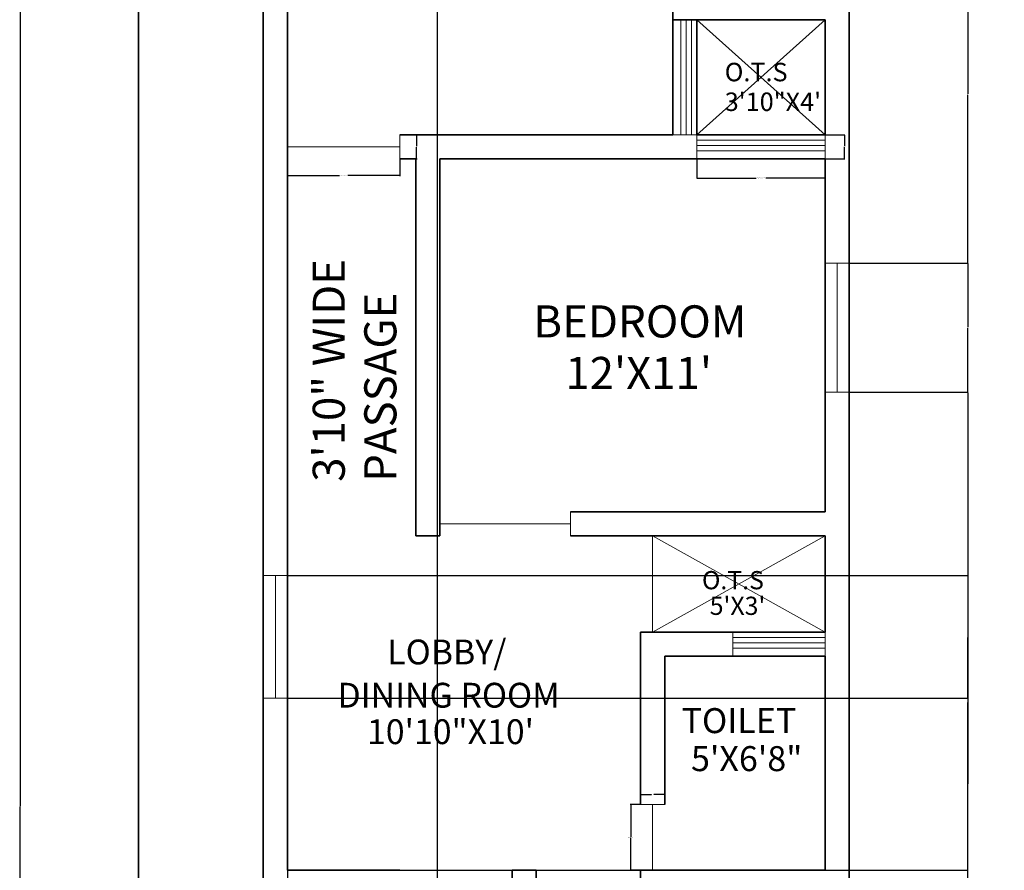
# Model space of a CAD drawing. Units: feet. Extents: x 2100 to 2836, y 2433 to 3396.
# Tile 7 of 12: x 2100 to 2468, y 2906 to 3224. Entities that reach past the tile are written whole.
import ezdxf

# ---------------------------------------------------------------- set-up
doc = ezdxf.new("R2010")
doc.units = ezdxf.units.FT
for name, color, linetype, lineweight in [('A-ANNO-DIMS', 2, 'Continuous', 18), ('A-ANNO-TTLB', 7, 'Continuous', 35), ('A-AREA-IDEN', 7, 'Continuous', 18), ('A-DOOR', 3, 'Continuous', 18), ('A-FLOR-OPEN', 8, 'Continuous', 13), ('A-GLAZ', 4, 'Continuous', 18), ('A-WALL', 7, 'Continuous', 35)]:
    doc.layers.add(name, color=color, linetype=linetype, lineweight=lineweight)
doc.styles.get("Standard").update_dxf_attribs({"font": 'arial.ttf'})
doc.dimstyles.get("Standard").update_dxf_attribs({"dimtxt": 0.18, "dimasz": 0.18, "dimexe": 0.18, "dimexo": 0.0625, "dimgap": 0.09, "dimtad": 0, "dimtih": 1, "dimtoh": 1, "dimdec": 4, "dimzin": 0, "dimdsep": 46, "dimtxsty": 'Standard', "dimcen": 0.09, "dimadec": 0, "dimazin": 0, "dimtfac": 1, "dimtdec": 4, "dimtofl": 0, "dimtmove": 0, "dimatfit": 3, "dimfxl": 1, "dimtolj": 1, "dimtzin": 0, "dimarcsym": 0})

# ---------------------------------------------------------------- blocks, each defined once
blk = doc.blocks.new('OTS-MARK-REAR')
for p, q in [((48, 0), (0, 43)), ((0, 0), (48, 43))]:
    blk.add_line(p, q)
blk = doc.blocks.new('OTS-MARK-LOBBY')
for p, q in [((0, 36), (64.5, 0)), ((0, 0), (64.5, 36))]:
    blk.add_line(p, q)
blk = doc.blocks.new('WIN-TOILET-OTS')
for p, q in [((0, 9), (0, 0)), ((34.5, 9), (34.5, 0)), ((34.5, 7), (0, 7)), ((34.5, 5), (0, 5)), ((34.5, 3), (0, 3))]:
    blk.add_line(p, q)
blk = doc.blocks.new('WIN-BEDROOM-OTS')
for p, q in [((0, 9), (0, 0)), ((48, 9), (48, 0)), ((0, 7), (48, 7)), ((0, 5), (48, 5)), ((0, 3), (48, 3))]:
    blk.add_line(p, q)
blk = doc.blocks.new('WIN-REAR-BEDROOM-OTS')
for p, q in [((3, 43), (3, 0)), ((5, 43), (5, 0)), ((7, 43), (7, 0)), ((0, 0), (9, 0))]:
    blk.add_line(p, q)
blk = doc.blocks.new('DOOR-LOBBY-TOILET')
for p, q in [((0, 24.62), (9, 24.62)), ((4.5, 24.62), (4.5, 0))]:
    blk.add_line(p, q)
blk = doc.blocks.new('DOOR-BEDROOM-LOBBY')
for p, q in [((48.78, 9), (48.78, 0)), ((48.78, 4.5), (0, 4.5))]:
    blk.add_line(p, q)
blk = doc.blocks.new('DOOR-PASSAGE')
for p, q in [((42, 0), (42, 9)), ((42, 4.5), (0, 4.5))]:
    blk.add_line(p, q)
blk = doc.blocks.new('*D16')
at = {"layer": 'A-ANNO-DIMS', "color": 0, "lineweight": -2, "transparency": 16777216}
for p, q in [((2199.69, 3171.74), (2199.69, 3165.32)), ((2241.69, 3171.74), (2241.69, 3165.32)), ((2199.87, 3165.5), (2219.11, 3165.5)), ((2241.51, 3165.5), (2222.26, 3165.5))]:
    blk.add_line(p, q, dxfattribs=at)
at = {"layer": 'A-ANNO-DIMS', "color": 0, "transparency": 16777216}
for points in [[(2199.87, 3165.53), (2199.87, 3165.47), (2199.69, 3165.5)], [(2241.51, 3165.53), (2241.51, 3165.47), (2241.69, 3165.5)]]:
    blk.add_solid(points, dxfattribs=at)
at = {"layer": 'Defpoints', "color": 0, "transparency": 16777216}
for p in [(2199.69, 3171.8), (2241.69, 3171.8), (2241.69, 3165.5)]:
    blk.add_point(p, dxfattribs=at)
at = {"layer": 'A-ANNO-DIMS', "color": 0, "transparency": 16777216, "insert": (2220.69, 3165.5), "char_height": 0.18, "attachment_point": 5}
blk.add_mtext('\\A1;PASSAGE DOOR 42 TYP.', dxfattribs=at)
blk = doc.blocks.new('*D17')
at = {"layer": 'A-ANNO-DIMS', "color": 0, "lineweight": -2, "transparency": 16777216}
for p, q in [((2241.75, 3180.8), (2248.17, 3180.8)), ((2247.99, 3180.62), (2247.99, 3176.48)), ((2247.99, 3171.98), (2247.99, 3176.12)), ((2241.75, 3171.8), (2248.17, 3171.8))]:
    blk.add_line(p, q, dxfattribs=at)
at = {"layer": 'A-ANNO-DIMS', "color": 0, "transparency": 16777216}
for points in [[(2247.96, 3180.62), (2248.02, 3180.62), (2247.99, 3180.8)], [(2247.96, 3171.98), (2248.02, 3171.98), (2247.99, 3171.8)]]:
    blk.add_solid(points, dxfattribs=at)
at = {"layer": 'Defpoints', "color": 0, "transparency": 16777216}
for p in [(2241.69, 3180.8), (2247.99, 3180.8), (2241.69, 3171.8)]:
    blk.add_point(p, dxfattribs=at)
at = {"layer": 'A-ANNO-DIMS', "color": 0, "transparency": 16777216, "insert": (2247.99, 3176.3), "char_height": 0.18, "attachment_point": 5}
blk.add_mtext('\\A1;9 TYP.', dxfattribs=at)
blk = doc.blocks.new('*D26')
at = {"layer": 'A-ANNO-DIMS', "color": 0, "lineweight": -2, "transparency": 16777216}
for p, q in [((2352.69, 3171.74), (2352.69, 3164.42)), ((2400.69, 3171.74), (2400.69, 3164.42)), ((2352.87, 3164.6), (2374.89, 3164.6)), ((2400.51, 3164.6), (2378.48, 3164.6))]:
    blk.add_line(p, q, dxfattribs=at)
at = {"layer": 'A-ANNO-DIMS', "color": 0, "transparency": 16777216}
for points in [[(2352.87, 3164.63), (2352.87, 3164.57), (2352.69, 3164.6)], [(2400.51, 3164.63), (2400.51, 3164.57), (2400.69, 3164.6)]]:
    blk.add_solid(points, dxfattribs=at)
at = {"layer": 'Defpoints', "color": 0, "transparency": 16777216}
for p in [(2352.69, 3171.8), (2400.69, 3171.8), (2400.69, 3164.6)]:
    blk.add_point(p, dxfattribs=at)
at = {"layer": 'A-ANNO-DIMS', "color": 0, "transparency": 16777216, "insert": (2376.69, 3164.6), "char_height": 0.18, "attachment_point": 5}
blk.add_mtext('\\A1;BEDROOM WINDOW 48 TYP.', dxfattribs=at)
blk = doc.blocks.new('*D27')
at = {"layer": 'A-ANNO-DIMS', "color": 0, "lineweight": -2, "transparency": 16777216}
for p, q in [((2400.75, 3180.8), (2408.07, 3180.8)), ((2407.89, 3180.62), (2407.89, 3176.48)), ((2407.89, 3171.98), (2407.89, 3176.12)), ((2400.75, 3171.8), (2408.07, 3171.8))]:
    blk.add_line(p, q, dxfattribs=at)
at = {"layer": 'A-ANNO-DIMS', "color": 0, "transparency": 16777216}
for points in [[(2407.86, 3180.62), (2407.92, 3180.62), (2407.89, 3180.8)], [(2407.86, 3171.98), (2407.92, 3171.98), (2407.89, 3171.8)]]:
    blk.add_solid(points, dxfattribs=at)
at = {"layer": 'Defpoints', "color": 0, "transparency": 16777216}
for p in [(2400.69, 3180.8), (2407.89, 3180.8), (2400.69, 3171.8)]:
    blk.add_point(p, dxfattribs=at)
at = {"layer": 'A-ANNO-DIMS', "color": 0, "transparency": 16777216, "insert": (2407.89, 3176.3), "char_height": 0.18, "attachment_point": 5}
blk.add_mtext('\\A1;9 TYP.', dxfattribs=at)
blk = doc.blocks.new('*D32')
at = {"layer": 'A-ANNO-DIMS', "color": 0, "lineweight": -2, "transparency": 16777216}
for p, q in [((2331.62, 2930.42), (2327.81, 2930.42)), ((2327.99, 2930.24), (2327.99, 2918.29)), ((2327.99, 2905.98), (2327.99, 2917.93)), ((2331.62, 2905.8), (2327.81, 2905.8))]:
    blk.add_line(p, q, dxfattribs=at)
at = {"layer": 'A-ANNO-DIMS', "color": 0, "transparency": 16777216}
for points in [[(2327.96, 2930.24), (2328.02, 2930.24), (2327.99, 2930.42)], [(2327.96, 2905.98), (2328.02, 2905.98), (2327.99, 2905.8)]]:
    blk.add_solid(points, dxfattribs=at)
at = {"layer": 'Defpoints', "color": 0, "transparency": 16777216}
for p in [(2327.99, 2930.42), (2331.69, 2930.42), (2331.69, 2905.8)]:
    blk.add_point(p, dxfattribs=at)
at = {"layer": 'A-ANNO-DIMS', "color": 0, "transparency": 16777216, "insert": (2327.99, 2918.11), "char_height": 0.18, "attachment_point": 5}
blk.add_mtext('\\A1;WC DOOR 25 TYP.', dxfattribs=at)
blk = doc.blocks.new('*D33')
at = {"layer": 'A-ANNO-DIMS', "color": 0, "lineweight": -2, "transparency": 16777216}
for p, q in [((2331.69, 2930.48), (2331.69, 2934.29)), ((2331.87, 2934.11), (2335.73, 2934.11)), ((2340.51, 2934.11), (2336.64, 2934.11)), ((2340.69, 2930.48), (2340.69, 2934.29))]:
    blk.add_line(p, q, dxfattribs=at)
at = {"layer": 'A-ANNO-DIMS', "color": 0, "transparency": 16777216}
for points in [[(2331.87, 2934.14), (2331.87, 2934.08), (2331.69, 2934.11)], [(2340.51, 2934.14), (2340.51, 2934.08), (2340.69, 2934.11)]]:
    blk.add_solid(points, dxfattribs=at)
at = {"layer": 'Defpoints', "color": 0, "transparency": 16777216}
for p in [(2340.69, 2934.11), (2331.69, 2930.42), (2340.69, 2930.42)]:
    blk.add_point(p, dxfattribs=at)
at = {"layer": 'A-ANNO-DIMS', "color": 0, "transparency": 16777216, "insert": (2336.19, 2934.11), "char_height": 0.18, "attachment_point": 5}
blk.add_mtext('\\A1;9 TYP.', dxfattribs=at)
blk = doc.blocks.new('*D41')
at = {"layer": 'A-ANNO-DIMS', "color": 0, "lineweight": -2, "transparency": 16777216}
for p, q in [((2190.62, 3321.8), (2099.65, 3321.8)), ((2099.83, 3321.62), (2099.83, 2929.96)), ((2099.83, 2537.94), (2099.83, 2929.6)), ((2190.62, 2537.76), (2099.65, 2537.76))]:
    blk.add_line(p, q, dxfattribs=at)
at = {"layer": 'A-ANNO-DIMS', "color": 0, "transparency": 16777216}
for points in [[(2099.8, 3321.62), (2099.86, 3321.62), (2099.83, 3321.8)], [(2099.8, 2537.94), (2099.86, 2537.94), (2099.83, 2537.76)]]:
    blk.add_solid(points, dxfattribs=at)
at = {"layer": 'Defpoints', "color": 0, "transparency": 16777216}
for p in [(2099.83, 3321.8), (2190.69, 3321.8), (2190.69, 2537.76)]:
    blk.add_point(p, dxfattribs=at)
at = {"layer": 'A-ANNO-DIMS', "color": 0, "transparency": 16777216, "insert": (2099.83, 2929.78), "char_height": 0.18, "attachment_point": 5}
blk.add_mtext('\\A1;784', dxfattribs=at)
blk = doc.blocks.new('*D44')
at = {"layer": 'A-ANNO-DIMS', "color": 0, "lineweight": -2, "transparency": 16777216}
for p, q in [((2199.69, 3312.74), (2199.69, 2433.01)), ((2255.63, 3312.74), (2255.63, 2433.01)), ((2199.87, 2433.19), (2227.26, 2433.19)), ((2255.45, 2433.19), (2228.05, 2433.19))]:
    blk.add_line(p, q, dxfattribs=at)
at = {"layer": 'A-ANNO-DIMS', "color": 0, "transparency": 16777216}
for points in [[(2199.87, 2433.22), (2199.87, 2433.16), (2199.69, 2433.19)], [(2255.45, 2433.22), (2255.45, 2433.16), (2255.63, 2433.19)]]:
    blk.add_solid(points, dxfattribs=at)
at = {"layer": 'Defpoints', "color": 0, "transparency": 16777216}
for p in [(2199.69, 3312.8), (2255.63, 3312.8), (2255.63, 2433.19)]:
    blk.add_point(p, dxfattribs=at)
at = {"layer": 'A-ANNO-DIMS', "color": 0, "transparency": 16777216, "insert": (2227.66, 2433.19), "char_height": 0.18, "attachment_point": 5}
blk.add_mtext('\\A1;55.94', dxfattribs=at)
blk = doc.blocks.new('*D48')
at = {"layer": 'A-ANNO-DIMS', "color": 0, "lineweight": -2, "transparency": 16777216}
for p, q in [((2409.75, 3259.04), (2454.12, 3259.04)), ((2453.94, 3258.86), (2453.94, 3196.12)), ((2453.94, 3133.01), (2453.94, 3195.75)), ((2409.75, 3132.83), (2454.12, 3132.83))]:
    blk.add_line(p, q, dxfattribs=at)
at = {"layer": 'A-ANNO-DIMS', "color": 0, "transparency": 16777216}
for points in [[(2453.91, 3258.86), (2453.97, 3258.86), (2453.94, 3259.04)], [(2453.91, 3133.01), (2453.97, 3133.01), (2453.94, 3132.83)]]:
    blk.add_solid(points, dxfattribs=at)
at = {"layer": 'Defpoints', "color": 0, "transparency": 16777216}
for p in [(2409.69, 3259.04), (2409.69, 3132.83), (2453.94, 3132.83)]:
    blk.add_point(p, dxfattribs=at)
at = {"layer": 'A-ANNO-DIMS', "color": 0, "transparency": 16777216, "insert": (2453.94, 3195.94), "char_height": 0.18, "attachment_point": 5}
blk.add_mtext('\\A1;126.2', dxfattribs=at)
blk = doc.blocks.new('*D49')
at = {"layer": 'A-ANNO-DIMS', "color": 0, "lineweight": -2, "transparency": 16777216}
for p, q in [((2409.75, 3132.83), (2454.12, 3132.83)), ((2453.94, 3132.65), (2453.94, 3108.87)), ((2453.94, 3084.72), (2453.94, 3108.51)), ((2409.75, 3084.54), (2454.12, 3084.54))]:
    blk.add_line(p, q, dxfattribs=at)
at = {"layer": 'A-ANNO-DIMS', "color": 0, "transparency": 16777216}
for points in [[(2453.91, 3132.65), (2453.97, 3132.65), (2453.94, 3132.83)], [(2453.91, 3084.72), (2453.97, 3084.72), (2453.94, 3084.54)]]:
    blk.add_solid(points, dxfattribs=at)
at = {"layer": 'Defpoints', "color": 0, "transparency": 16777216}
for p in [(2409.69, 3132.83), (2409.69, 3084.54), (2453.94, 3084.54)]:
    blk.add_point(p, dxfattribs=at)
at = {"layer": 'A-ANNO-DIMS', "color": 0, "transparency": 16777216, "insert": (2453.94, 3108.69), "char_height": 0.18, "attachment_point": 5}
blk.add_mtext('\\A1;48.29', dxfattribs=at)
blk = doc.blocks.new('*D50')
at = {"layer": 'A-ANNO-DIMS', "color": 0, "lineweight": -2, "transparency": 16777216}
for p, q in [((2409.75, 3084.54), (2454.12, 3084.54)), ((2453.94, 3084.36), (2453.94, 2968.97)), ((2453.94, 2853.21), (2453.94, 2968.6)), ((2409.75, 2853.03), (2454.12, 2853.03))]:
    blk.add_line(p, q, dxfattribs=at)
at = {"layer": 'A-ANNO-DIMS', "color": 0, "transparency": 16777216}
for points in [[(2453.91, 3084.36), (2453.97, 3084.36), (2453.94, 3084.54)], [(2453.91, 2853.21), (2453.97, 2853.21), (2453.94, 2853.03)]]:
    blk.add_solid(points, dxfattribs=at)
at = {"layer": 'Defpoints', "color": 0, "transparency": 16777216}
for p in [(2409.69, 3084.54), (2409.69, 2853.03), (2453.94, 2853.03)]:
    blk.add_point(p, dxfattribs=at)
at = {"layer": 'A-ANNO-DIMS', "color": 0, "transparency": 16777216, "insert": (2453.94, 2968.78), "char_height": 0.18, "attachment_point": 5}
blk.add_mtext('\\A1;231.5', dxfattribs=at)
blk = doc.blocks.new('*D52')
at = {"layer": 'A-ANNO-DIMS', "color": 0, "lineweight": -2, "transparency": 16777216}
for p, q in [((2199.75, 2970.11), (2454.12, 2970.11)), ((2453.94, 2969.93), (2453.94, 2938.14)), ((2453.94, 2905.98), (2453.94, 2937.78)), ((2199.75, 2905.8), (2454.12, 2905.8))]:
    blk.add_line(p, q, dxfattribs=at)
at = {"layer": 'A-ANNO-DIMS', "color": 0, "transparency": 16777216}
for points in [[(2453.91, 2969.93), (2453.97, 2969.93), (2453.94, 2970.11)], [(2453.91, 2905.98), (2453.97, 2905.98), (2453.94, 2905.8)]]:
    blk.add_solid(points, dxfattribs=at)
at = {"layer": 'Defpoints', "color": 0, "transparency": 16777216}
for p in [(2199.69, 2970.11), (2453.94, 2970.11), (2199.69, 2905.8)]:
    blk.add_point(p, dxfattribs=at)
at = {"layer": 'A-ANNO-DIMS', "color": 0, "transparency": 16777216, "insert": (2453.94, 2937.96), "char_height": 0.18, "attachment_point": 5}
blk.add_mtext('\\A1;64.31', dxfattribs=at)
blk = doc.blocks.new('*D53')
at = {"layer": 'A-ANNO-DIMS', "color": 0, "lineweight": -2, "transparency": 16777216}
for p, q in [((2199.75, 3016.03), (2454.12, 3016.03)), ((2453.94, 3015.85), (2453.94, 2993.26)), ((2453.94, 2970.29), (2453.94, 2992.89)), ((2199.75, 2970.11), (2454.12, 2970.11))]:
    blk.add_line(p, q, dxfattribs=at)
at = {"layer": 'A-ANNO-DIMS', "color": 0, "transparency": 16777216}
for points in [[(2453.91, 3015.85), (2453.97, 3015.85), (2453.94, 3016.03)], [(2453.91, 2970.29), (2453.97, 2970.29), (2453.94, 2970.11)]]:
    blk.add_solid(points, dxfattribs=at)
at = {"layer": 'Defpoints', "color": 0, "transparency": 16777216}
for p in [(2199.69, 3016.03), (2453.94, 3016.03), (2199.69, 2970.11)]:
    blk.add_point(p, dxfattribs=at)
at = {"layer": 'A-ANNO-DIMS', "color": 0, "transparency": 16777216, "insert": (2453.94, 2993.07), "char_height": 0.18, "attachment_point": 5}
blk.add_mtext('\\A1;45.92', dxfattribs=at)

msp = doc.modelspace()

# ---------------------------------------------------------------- linework, layer by layer
at = {"layer": 'A-ANNO-TTLB'}
msp.add_lwpolyline([(2144.0848, 3351.6245), (2791.0561, 3351.6245), (2791.0561, 2477.4373), (2144.0848, 2477.4373)], close=True, dxfattribs=at)
at = {"layer": 'A-FLOR-OPEN'}
msp.add_line((2336.1857, 2994.8031), (2336.1857, 3030.8031), dxfattribs=at)
at = {"layer": 'A-GLAZ'}
for p, q in [((2400.6857, 3132.8348), (2409.6857, 3132.8348)), ((2405.1857, 3084.5411), (2405.1857, 3132.8348)), ((2400.6857, 3084.5411), (2409.6857, 3084.5411)), ((2190.6857, 3016.035), (2199.6857, 3016.035)), ((2195.1857, 2970.1128), (2195.1857, 3016.035)), ((2190.6857, 2970.1128), (2199.6857, 2970.1128))]:
    msp.add_line(p, q, dxfattribs=at)
at = {"layer": 'A-WALL'}
for p, q in [((2190.6857, 2593.755), (2190.6857, 3321.8031)), ((2409.6857, 3321.8031), (2409.6857, 3171.8031)), ((2199.6857, 2905.8031), (2199.6857, 3312.8031)), ((2343.6857, 3260.1235), (2343.6857, 3180.8031)), ((2400.6857, 3223.8031), (2343.6857, 3223.8031)), ((2352.6857, 3223.8031), (2352.6857, 3180.8031)), ((2352.6857, 3223.8031), (2352.6857, 3180.8031)), ((2352.6857, 3223.8031), (2352.6857, 3180.8031)), ((2352.6857, 3223.8031), (2400.6857, 3223.8031)), ((2352.6857, 3223.8031), (2396.5765, 3223.8031)), ((2400.6857, 3223.8031), (2400.6857, 3180.8031)), ((2343.6857, 3180.8031), (2241.6857, 3180.8031)), ((2352.6857, 3180.8031), (2400.6857, 3180.8031)), ((2247.6857, 3171.8031), (2241.6857, 3171.8031)), ((2247.6857, 3171.8031), (2247.6857, 3039.8031)), ((2400.6857, 3171.8031), (2256.6857, 3171.8031)), ((2256.6857, 3171.8031), (2256.6857, 3030.8031)), ((2400.6857, 3039.8031), (2400.6857, 3171.8031)), ((2409.6857, 3171.8031), (2409.6857, 2987.2733)), ((2247.6857, 3039.8031), (2247.6857, 3030.8031)), ((2305.4641, 3039.8031), (2400.6857, 3039.8031)), ((2247.6857, 3030.8031), (2256.6857, 3030.8031)), ((2305.4641, 3030.8031), (2400.6857, 3030.8031)), ((2400.6857, 3030.8031), (2400.6857, 2994.8031)), ((2400.6857, 2994.8031), (2331.6857, 2994.8031)), ((2331.6857, 2994.8031), (2331.6857, 2930.4198)), ((2400.6857, 2985.8031), (2340.6857, 2985.8031)), ((2340.6857, 2985.8031), (2340.6857, 2930.4198)), ((2400.6857, 2905.8031), (2400.6857, 2985.8031)), ((2409.6857, 2987.2733), (2409.6857, 2891.1053)), ((2241.6857, 2905.8031), (2199.6857, 2905.8031)), ((2283.6857, 2905.8031), (2292.6857, 2905.8031)), ((2283.6857, 2810.8031), (2283.6857, 2905.8031)), ((2292.6857, 2801.8031), (2292.6857, 2905.8031)), ((2331.6857, 2905.8031), (2331.6857, 2896.8031)), ((2331.6857, 2905.8031), (2400.6857, 2905.8031))]:
    msp.add_line(p, q, dxfattribs=at)

# ---------------------------------------------------------------- block references
at = {"layer": 'A-DOOR'}
for name, p in [('DOOR-PASSAGE', (2199.6857, 3171.8031)), ('DOOR-BEDROOM-LOBBY', (2256.6857, 3030.8031)), ('DOOR-LOBBY-TOILET', (2331.6857, 2905.8031))]:
    msp.add_blockref(name, p, dxfattribs=at)
at = {"layer": 'A-FLOR-OPEN'}
for name, p in [('OTS-MARK-REAR', (2352.6857, 3180.8031)), ('OTS-MARK-LOBBY', (2336.1857, 2994.8031))]:
    msp.add_blockref(name, p, dxfattribs=at)
at = {"layer": 'A-GLAZ'}
for name, p in [('WIN-REAR-BEDROOM-OTS', (2343.6857, 3180.8031)), ('WIN-BEDROOM-OTS', (2352.6857, 3171.8031)), ('WIN-TOILET-OTS', (2366.1857, 2985.8031))]:
    msp.add_blockref(name, p, dxfattribs=at)

# ---------------------------------------------------------------- texts
at = {"layer": 'A-AREA-IDEN'}
for s, height, p in [('O.T.S', 6.90977, (2363.1223, 3200.7703)), ('3\'10"X4\'', 6.90977, (2363.1223, 3189.6704)), ('BEDROOM', 12, (2291.5872, 3105.0073)), ("12'X11'", 12, (2303.5571, 3085.7303)), ('O.T.S', 6.80645, (2354.6282, 3010.8676)), ("5'X3'", 6.80645, (2357.5254, 3001.2906)), ('LOBBY/', 9.27498, (2237.0096, 2982.7864)), ('DINING ROOM', 9.274981, (2218.3777, 2966.6248)), ('TOILET', 9.33724, (2347.0047, 2957.0883)), ('10\'10"X10\'', 9.27498, (2229.4306, 2952.9875)), ('5\'X6\'8"', 9.33724, (2350.5226, 2942.8877))]:
    msp.add_text(s, height=height, dxfattribs=at).set_placement(p)
for s, p in [('3\'10" WIDE ', (2221.1429, 3051.0405)), ('PASSAGE', (2240.4199, 3051.0405))]:
    msp.add_text(s, height=12, rotation=90, dxfattribs=at).set_placement(p)

# ---------------------------------------------------------------- dimensions: what is measured, and where the dimension line sits
at = {"layer": 'A-ANNO-DIMS'}
for base, p1, p2, override, picture, middle in [((2099.8348, 3321.8031), (2190.6857, 2537.755), (2190.6857, 3321.8031), {"dimdec": 0, "dimlfac": 1, "dimrnd": 0, "dimzin": 0, "dimdsep": 46, "dimlunit": 2}, '*D41', (2099.8348, 2929.7791)), ((2453.9357, 3132.8348), (2409.6857, 3259.0368), (2409.6857, 3132.8348), {"dimdec": 1, "dimlfac": 1, "dimrnd": 0, "dimzin": 0, "dimdsep": 46, "dimlunit": 2}, '*D48', (2453.9357, 3195.9358)), ((2453.9357, 3084.5411), (2409.6857, 3132.8348), (2409.6857, 3084.5411), {"dimdec": 2, "dimlfac": 1, "dimrnd": 0, "dimzin": 0, "dimdsep": 46, "dimlunit": 2}, '*D49', (2453.9357, 3108.688)), ((2453.9357, 2853.0255), (2409.6857, 3084.5411), (2409.6857, 2853.0255), {"dimdec": 1, "dimlfac": 1, "dimrnd": 0, "dimzin": 0, "dimdsep": 46, "dimlunit": 2}, '*D50', (2453.9357, 2968.7833)), ((2453.9357, 3016.035), (2199.6857, 2970.1128), (2199.6857, 3016.035), {"dimdec": 2, "dimlfac": 1, "dimrnd": 0, "dimzin": 0, "dimdsep": 46, "dimlunit": 2}, '*D53', (2453.9357, 2993.0739)), ((2453.9357, 2970.1128), (2199.6857, 2905.8031), (2199.6857, 2970.1128), {"dimdec": 2, "dimlfac": 1, "dimrnd": 0, "dimzin": 0, "dimdsep": 46, "dimlunit": 2}, '*D52', (2453.9357, 2937.9579))]:
    dim = msp.add_linear_dim(base=base, p1=p1, p2=p2, angle=90, dimstyle='Standard', override=override, dxfattribs=at)
    dim.commit()
    dim.dimension.update_dxf_attribs({"geometry": picture, "text_midpoint": middle})
dim = msp.add_linear_dim(base=(2255.625, 2433.1873), p1=(2199.6857, 3312.8031), p2=(2255.625, 3312.8031), dimstyle='Standard', override={"dimdec": 2, "dimlfac": 1, "dimrnd": 0, "dimzin": 0, "dimdsep": 46, "dimlunit": 2}, dxfattribs=at)
dim.commit()
dim.dimension.update_dxf_attribs({"geometry": '*D44', "text_midpoint": (2227.6554, 2433.1873)})
for base, p1, p2, text, picture, middle in [((2247.9857, 3180.8031), (2241.6857, 3171.8031), (2241.6857, 3180.8031), '<> TYP.', '*D17', (2247.9857, 3176.3031)), ((2407.8857, 3180.8031), (2400.6857, 3171.8031), (2400.6857, 3180.8031), '<> TYP.', '*D27', (2407.8857, 3176.3031)), ((2327.9932, 2930.4198), (2331.6857, 2905.8031), (2331.6857, 2930.4198), 'WC DOOR <> TYP.', '*D32', (2327.9932, 2918.1114))]:
    dim = msp.add_linear_dim(base=base, p1=p1, p2=p2, angle=90, text=text, dimstyle='Standard', override={"dimdec": 0, "dimlfac": 1, "dimrnd": 0, "dimzin": 0, "dimdsep": 46, "dimlunit": 2}, dxfattribs=at)
    dim.commit()
    dim.dimension.update_dxf_attribs({"geometry": picture, "text_midpoint": middle})
for base, p1, p2, text, picture, middle in [((2241.6857, 3165.5031), (2199.6857, 3171.8031), (2241.6857, 3171.8031), 'PASSAGE DOOR <> TYP.', '*D16', (2220.6857, 3165.5031)), ((2400.6857, 3164.6031), (2352.6857, 3171.8031), (2400.6857, 3171.8031), 'BEDROOM WINDOW <> TYP.', '*D26', (2376.6857, 3164.6031)), ((2340.6857, 2934.1123), (2331.6857, 2930.4198), (2340.6857, 2930.4198), '<> TYP.', '*D33', (2336.1857, 2934.1123))]:
    dim = msp.add_linear_dim(base=base, p1=p1, p2=p2, text=text, dimstyle='Standard', override={"dimdec": 0, "dimlfac": 1, "dimrnd": 0, "dimzin": 0, "dimdsep": 46, "dimlunit": 2}, dxfattribs=at)
    dim.commit()
    dim.dimension.update_dxf_attribs({"geometry": picture, "text_midpoint": middle})

doc.saveas('drawing.dxf')
